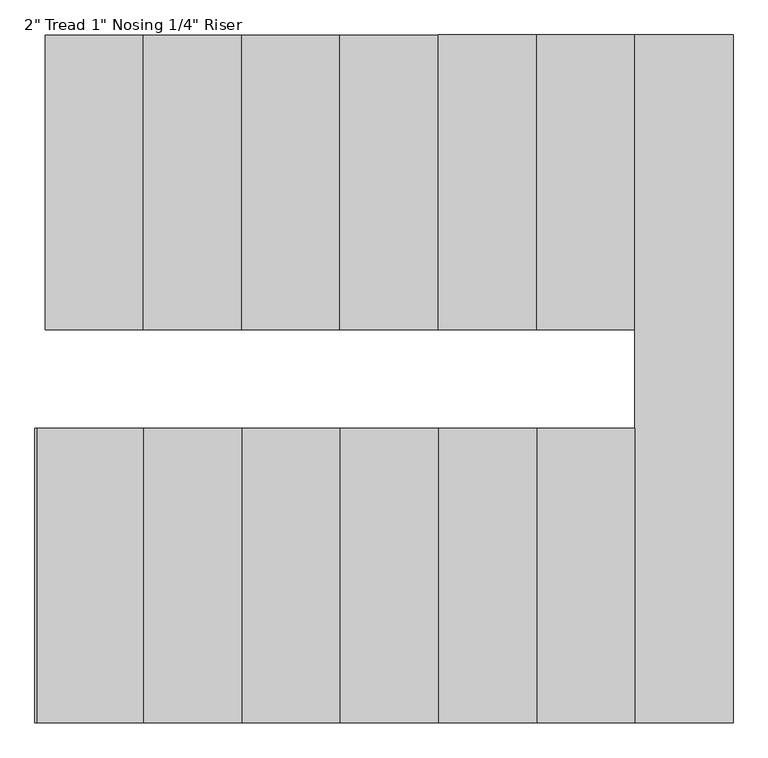
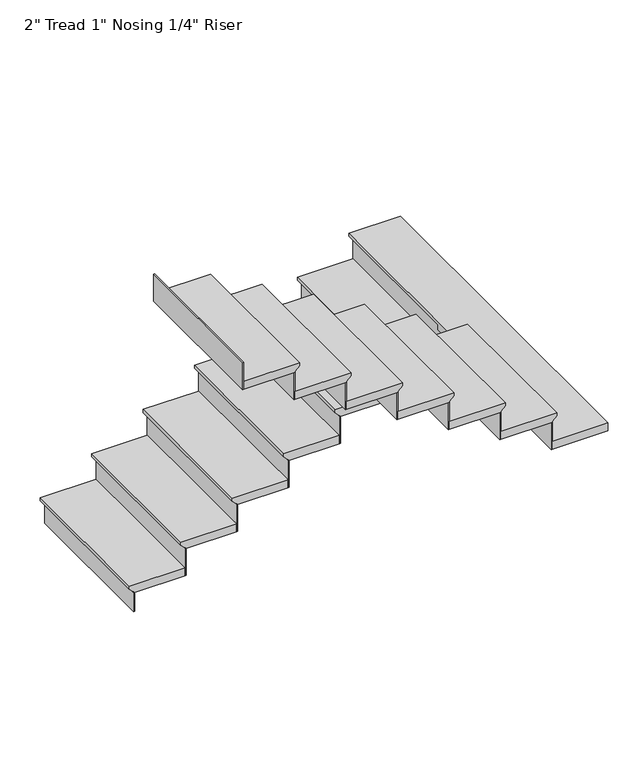
"""IFC4 building model written with IfcOpenShell, lengths in millimetres: stair flight geometry."""

from ifc_helpers import new_model, si_unit, origin, place, context, project, spatial, faceted_brep, source, transform, mapped, element, save


def stair_flight_65dd4c8f(model_context):
    return source(origin(), model_context, "Body", "Brep", [
        faceted_brep([(5003.8, 8661.4, 150.2833333), (5003.8, 8661.4, 169.3333333), (5003.8, 9575.8, 169.3333333), (5003.8, 9575.8, 150.2833333), (5029.2, 8661.4, 124.8833333), (5029.2, 9575.8, 124.8833333), (5334.0, 8661.4, 169.3333333), (5334.0, 9575.8, 169.3333333), (5029.2, 9575.8, 118.5333333), (5334.0, 9575.8, 118.5333333), (5334.0, 8661.4, 118.5333333), (5029.2, 8661.4, 118.5333333)], [[[0, 1, 2, 3]], [[4, 0, 3, 5]], [[2, 1, 6, 7]], [[8, 9, 10, 11]], [[2, 7, 9, 8, 5, 3]], [[8, 11, 4, 5]], [[6, 1, 0, 4, 11, 10]], [[7, 6, 10, 9]]]),
        faceted_brep([(5029.2, 8661.4, 118.5333333), (5029.2, 8661.4, 0.0), (5035.55, 8661.4, 0.0), (5035.55, 8661.4, 118.5333333), (5029.2, 9575.8, 118.5333333), (5035.55, 9575.8, 118.5333333), (5035.55, 9575.8, 0.0), (5029.2, 9575.8, 0.0)], [[[0, 1, 2, 3]], [[4, 5, 6, 7]], [[1, 0, 4, 7]], [[2, 1, 7, 6]], [[3, 2, 6, 5]], [[0, 3, 5, 4]]]),
        faceted_brep([(5334.0, 8661.4, 287.8666667), (5334.0, 8661.4, 118.5333333), (5340.35, 8661.4, 118.5333333), (5340.35, 8661.4, 287.8666667), (5334.0, 9575.8, 287.8666667), (5340.35, 9575.8, 287.8666667), (5340.35, 9575.8, 118.5333333), (5334.0, 9575.8, 118.5333333)], [[[0, 1, 2, 3]], [[4, 5, 6, 7]], [[1, 0, 4, 7]], [[2, 1, 7, 6]], [[3, 2, 6, 5]], [[0, 3, 5, 4]]]),
        faceted_brep([(5308.6, 9575.8, 338.6666667), (5308.6, 8661.4, 338.6666667), (5638.8, 8661.4, 338.6666667), (5638.8, 9575.8, 338.6666667), (5334.0, 9575.8, 287.8666667), (5638.8, 9575.8, 287.8666667), (5638.8, 8661.4, 287.8666667), (5334.0, 8661.4, 287.8666667), (5334.0, 9575.8, 294.2166667), (5308.6, 9575.8, 319.6166667), (5334.0, 8661.4, 294.2166667), (5308.6, 8661.4, 319.6166667)], [[[0, 1, 2, 3]], [[4, 5, 6, 7]], [[0, 3, 5, 4, 8, 9]], [[4, 7, 10, 8]], [[2, 1, 11, 10, 7, 6]], [[3, 2, 6, 5]], [[11, 1, 0, 9]], [[10, 11, 9, 8]]]),
        faceted_brep([(5638.8, 8661.4, 457.2), (5638.8, 8661.4, 287.8666667), (5645.15, 8661.4, 287.8666667), (5645.15, 8661.4, 457.2), (5638.8, 9575.8, 457.2), (5645.15, 9575.8, 457.2), (5645.15, 9575.8, 287.8666667), (5638.8, 9575.8, 287.8666667)], [[[0, 1, 2, 3]], [[4, 5, 6, 7]], [[1, 0, 4, 7]], [[2, 1, 7, 6]], [[3, 2, 6, 5]], [[0, 3, 5, 4]]]),
        faceted_brep([(5613.4, 9575.8, 508.0), (5613.4, 8661.4, 508.0), (5943.6, 8661.4, 508.0), (5943.6, 9575.8, 508.0), (5638.8, 9575.8, 457.2), (5943.6, 9575.8, 457.2), (5943.6, 8661.4, 457.2), (5638.8, 8661.4, 457.2), (5638.8, 9575.8, 463.55), (5613.4, 9575.8, 488.95), (5638.8, 8661.4, 463.55), (5613.4, 8661.4, 488.95)], [[[0, 1, 2, 3]], [[4, 5, 6, 7]], [[0, 3, 5, 4, 8, 9]], [[4, 7, 10, 8]], [[2, 1, 11, 10, 7, 6]], [[3, 2, 6, 5]], [[11, 1, 0, 9]], [[10, 11, 9, 8]]]),
        faceted_brep([(5943.6, 8661.4, 626.5333333), (5943.6, 8661.4, 457.2), (5949.95, 8661.4, 457.2), (5949.95, 8661.4, 626.5333333), (5943.6, 9575.8, 626.5333333), (5949.95, 9575.8, 626.5333333), (5949.95, 9575.8, 457.2), (5943.6, 9575.8, 457.2)], [[[0, 1, 2, 3]], [[4, 5, 6, 7]], [[1, 0, 4, 7]], [[2, 1, 7, 6]], [[3, 2, 6, 5]], [[0, 3, 5, 4]]]),
        faceted_brep([(5918.2, 9575.8, 677.3333333), (5918.2, 8661.4, 677.3333333), (6248.4, 8661.4, 677.3333333), (6248.4, 9575.8, 677.3333333), (5943.6, 9575.8, 626.5333333), (6248.4, 9575.8, 626.5333333), (6248.4, 8661.4, 626.5333333), (5943.6, 8661.4, 626.5333333), (5943.6, 9575.8, 632.8833333), (5918.2, 9575.8, 658.2833333), (5943.6, 8661.4, 632.8833333), (5918.2, 8661.4, 658.2833333)], [[[0, 1, 2, 3]], [[4, 5, 6, 7]], [[0, 3, 5, 4, 8, 9]], [[4, 7, 10, 8]], [[2, 1, 11, 10, 7, 6]], [[3, 2, 6, 5]], [[11, 1, 0, 9]], [[10, 11, 9, 8]]]),
        faceted_brep([(6248.4, 8661.4, 795.8666667), (6248.4, 8661.4, 626.5333333), (6254.75, 8661.4, 626.5333333), (6254.75, 8661.4, 795.8666667), (6248.4, 9575.8, 795.8666667), (6254.75, 9575.8, 795.8666667), (6254.75, 9575.8, 626.5333333), (6248.4, 9575.8, 626.5333333)], [[[0, 1, 2, 3]], [[4, 5, 6, 7]], [[1, 0, 4, 7]], [[2, 1, 7, 6]], [[3, 2, 6, 5]], [[0, 3, 5, 4]]]),
        faceted_brep([(6223.0, 9575.8, 846.6666667), (6223.0, 8661.4, 846.6666667), (6553.2, 8661.4, 846.6666667), (6553.2, 9575.8, 846.6666667), (6248.4, 9575.8, 795.8666667), (6553.2, 9575.8, 795.8666667), (6553.2, 8661.4, 795.8666667), (6248.4, 8661.4, 795.8666667), (6248.4, 9575.8, 802.2166667), (6223.0, 9575.8, 827.6166667), (6248.4, 8661.4, 802.2166667), (6223.0, 8661.4, 827.6166667)], [[[0, 1, 2, 3]], [[4, 5, 6, 7]], [[0, 3, 5, 4, 8, 9]], [[4, 7, 10, 8]], [[2, 1, 11, 10, 7, 6]], [[3, 2, 6, 5]], [[11, 1, 0, 9]], [[10, 11, 9, 8]]]),
        faceted_brep([(6553.2, 8661.4, 965.2), (6553.2, 8661.4, 795.8666667), (6559.55, 8661.4, 795.8666667), (6559.55, 8661.4, 965.2), (6553.2, 9575.8, 965.2), (6559.55, 9575.8, 965.2), (6559.55, 9575.8, 795.8666667), (6553.2, 9575.8, 795.8666667)], [[[0, 1, 2, 3]], [[4, 5, 6, 7]], [[1, 0, 4, 7]], [[2, 1, 7, 6]], [[3, 2, 6, 5]], [[0, 3, 5, 4]]]),
        faceted_brep([(6527.8, 9575.8, 1016.0), (6527.8, 8661.4, 1016.0), (6858.0, 8661.4, 1016.0), (6858.0, 9575.8, 1016.0), (6553.2, 9575.8, 965.2), (6858.0, 9575.8, 965.2), (6858.0, 8661.4, 965.2), (6553.2, 8661.4, 965.2), (6553.2, 9575.8, 971.55), (6527.8, 9575.8, 996.95), (6553.2, 8661.4, 971.55), (6527.8, 8661.4, 996.95)], [[[0, 1, 2, 3]], [[4, 5, 6, 7]], [[0, 3, 5, 4, 8, 9]], [[4, 7, 10, 8]], [[2, 1, 11, 10, 7, 6]], [[3, 2, 6, 5]], [[11, 1, 0, 9]], [[10, 11, 9, 8]]]),
        faceted_brep([(6858.0, 8661.4, 1134.5333333), (6858.0, 8661.4, 965.2), (6864.35, 8661.4, 965.2), (6864.35, 8661.4, 1134.5333333), (6858.0, 9575.8, 1134.5333333), (6864.35, 9575.8, 1134.5333333), (6864.35, 9575.8, 965.2), (6858.0, 9575.8, 965.2)], [[[0, 1, 2, 3]], [[4, 5, 6, 7]], [[1, 0, 4, 7]], [[2, 1, 7, 6]], [[3, 2, 6, 5]], [[0, 3, 5, 4]]]),
        faceted_brep([(6807.2, 7442.2, 1185.3333333), (7137.4, 7442.2, 1185.3333333), (7137.4, 9575.8, 1185.3333333), (6832.6, 9575.8, 1185.3333333), (6832.6, 8356.6, 1185.3333333), (6807.2, 8356.6, 1185.3333333), (7137.4, 7442.2, 1134.5333333), (6807.2, 7442.2, 1134.5333333), (6807.2, 8356.6, 1134.5333333), (6832.6, 8356.6, 1134.5333333), (6832.6, 8661.4, 1134.5333333), (6858.0, 8661.4, 1134.5333333), (6858.0, 9575.8, 1134.5333333), (7137.4, 9575.8, 1134.5333333), (6858.0, 9575.8, 1140.8833333), (6832.6, 9575.8, 1166.2833333), (6858.0, 8661.4, 1140.8833333), (6832.6, 8661.4, 1166.2833333)], [[[0, 1, 2, 3, 4, 5]], [[6, 7, 8, 9, 10, 11, 12, 13]], [[1, 0, 7, 6]], [[2, 1, 6, 13]], [[3, 2, 13, 12, 14, 15]], [[12, 11, 16, 14]], [[11, 10, 17, 16]], [[4, 3, 15, 17, 10, 9]], [[5, 4, 9, 8]], [[0, 5, 8, 7]], [[15, 14, 16, 17]]]),
        faceted_brep([(6807.2, 8356.6, 1303.8666667), (6807.2, 8356.6, 1134.5333333), (6800.85, 8356.6, 1134.5333333), (6800.85, 8356.6, 1303.8666667), (6807.2, 7442.2, 1303.8666667), (6800.85, 7442.2, 1303.8666667), (6800.85, 7442.2, 1134.5333333), (6807.2, 7442.2, 1134.5333333)], [[[0, 1, 2, 3]], [[4, 5, 6, 7]], [[1, 0, 4, 7]], [[2, 1, 7, 6]], [[3, 2, 6, 5]], [[0, 3, 5, 4]]]),
        faceted_brep([(6832.6, 7442.2, 1354.6666667), (6832.6, 8356.6, 1354.6666667), (6502.4, 8356.6, 1354.6666667), (6502.4, 7442.2, 1354.6666667), (6807.2, 7442.2, 1303.8666667), (6502.4, 7442.2, 1303.8666667), (6502.4, 8356.6, 1303.8666667), (6807.2, 8356.6, 1303.8666667), (6807.2, 7442.2, 1310.2166667), (6832.6, 7442.2, 1335.6166667), (6807.2, 8356.6, 1310.2166667), (6832.6, 8356.6, 1335.6166667)], [[[0, 1, 2, 3]], [[4, 5, 6, 7]], [[0, 3, 5, 4, 8, 9]], [[4, 7, 10, 8]], [[2, 1, 11, 10, 7, 6]], [[3, 2, 6, 5]], [[11, 1, 0, 9]], [[10, 11, 9, 8]]]),
        faceted_brep([(6502.4, 8356.6, 1473.2), (6502.4, 8356.6, 1303.8666667), (6496.05, 8356.6, 1303.8666667), (6496.05, 8356.6, 1473.2), (6502.4, 7442.2, 1473.2), (6496.05, 7442.2, 1473.2), (6496.05, 7442.2, 1303.8666667), (6502.4, 7442.2, 1303.8666667)], [[[0, 1, 2, 3]], [[4, 5, 6, 7]], [[1, 0, 4, 7]], [[2, 1, 7, 6]], [[3, 2, 6, 5]], [[0, 3, 5, 4]]]),
        faceted_brep([(6527.8, 7442.2, 1524.0), (6527.8, 8356.6, 1524.0), (6197.6, 8356.6, 1524.0), (6197.6, 7442.2, 1524.0), (6502.4, 7442.2, 1473.2), (6197.6, 7442.2, 1473.2), (6197.6, 8356.6, 1473.2), (6502.4, 8356.6, 1473.2), (6502.4, 7442.2, 1479.55), (6527.8, 7442.2, 1504.95), (6502.4, 8356.6, 1479.55), (6527.8, 8356.6, 1504.95)], [[[0, 1, 2, 3]], [[4, 5, 6, 7]], [[0, 3, 5, 4, 8, 9]], [[4, 7, 10, 8]], [[2, 1, 11, 10, 7, 6]], [[3, 2, 6, 5]], [[11, 1, 0, 9]], [[10, 11, 9, 8]]]),
        faceted_brep([(6197.6, 8356.6, 1642.5333333), (6197.6, 8356.6, 1473.2), (6191.25, 8356.6, 1473.2), (6191.25, 8356.6, 1642.5333333), (6197.6, 7442.2, 1642.5333333), (6191.25, 7442.2, 1642.5333333), (6191.25, 7442.2, 1473.2), (6197.6, 7442.2, 1473.2)], [[[0, 1, 2, 3]], [[4, 5, 6, 7]], [[1, 0, 4, 7]], [[2, 1, 7, 6]], [[3, 2, 6, 5]], [[0, 3, 5, 4]]]),
        faceted_brep([(6223.0, 7442.2, 1693.3333333), (6223.0, 8356.6, 1693.3333333), (5892.8, 8356.6, 1693.3333333), (5892.8, 7442.2, 1693.3333333), (6197.6, 7442.2, 1642.5333333), (5892.8, 7442.2, 1642.5333333), (5892.8, 8356.6, 1642.5333333), (6197.6, 8356.6, 1642.5333333), (6197.6, 7442.2, 1648.8833333), (6223.0, 7442.2, 1674.2833333), (6197.6, 8356.6, 1648.8833333), (6223.0, 8356.6, 1674.2833333)], [[[0, 1, 2, 3]], [[4, 5, 6, 7]], [[0, 3, 5, 4, 8, 9]], [[4, 7, 10, 8]], [[2, 1, 11, 10, 7, 6]], [[3, 2, 6, 5]], [[11, 1, 0, 9]], [[10, 11, 9, 8]]]),
        faceted_brep([(5892.8, 8356.6, 1811.8666667), (5892.8, 8356.6, 1642.5333333), (5886.45, 8356.6, 1642.5333333), (5886.45, 8356.6, 1811.8666667), (5892.8, 7442.2, 1811.8666667), (5886.45, 7442.2, 1811.8666667), (5886.45, 7442.2, 1642.5333333), (5892.8, 7442.2, 1642.5333333)], [[[0, 1, 2, 3]], [[4, 5, 6, 7]], [[1, 0, 4, 7]], [[2, 1, 7, 6]], [[3, 2, 6, 5]], [[0, 3, 5, 4]]]),
        faceted_brep([(5918.2, 7442.2, 1862.6666667), (5918.2, 8356.6, 1862.6666667), (5588.0, 8356.6, 1862.6666667), (5588.0, 7442.2, 1862.6666667), (5892.8, 7442.2, 1811.8666667), (5588.0, 7442.2, 1811.8666667), (5588.0, 8356.6, 1811.8666667), (5892.8, 8356.6, 1811.8666667), (5892.8, 7442.2, 1818.2166667), (5918.2, 7442.2, 1843.6166667), (5892.8, 8356.6, 1818.2166667), (5918.2, 8356.6, 1843.6166667)], [[[0, 1, 2, 3]], [[4, 5, 6, 7]], [[0, 3, 5, 4, 8, 9]], [[4, 7, 10, 8]], [[2, 1, 11, 10, 7, 6]], [[3, 2, 6, 5]], [[11, 1, 0, 9]], [[10, 11, 9, 8]]]),
        faceted_brep([(5588.0, 8356.6, 1981.2), (5588.0, 8356.6, 1811.8666667), (5581.65, 8356.6, 1811.8666667), (5581.65, 8356.6, 1981.2), (5588.0, 7442.2, 1981.2), (5581.65, 7442.2, 1981.2), (5581.65, 7442.2, 1811.8666667), (5588.0, 7442.2, 1811.8666667)], [[[0, 1, 2, 3]], [[4, 5, 6, 7]], [[1, 0, 4, 7]], [[2, 1, 7, 6]], [[3, 2, 6, 5]], [[0, 3, 5, 4]]]),
        faceted_brep([(5613.4, 7442.2, 2032.0), (5613.4, 8356.6, 2032.0), (5283.2, 8356.6, 2032.0), (5283.2, 7442.2, 2032.0), (5588.0, 7442.2, 1981.2), (5283.2, 7442.2, 1981.2), (5283.2, 8356.6, 1981.2), (5588.0, 8356.6, 1981.2), (5588.0, 7442.2, 1987.55), (5613.4, 7442.2, 2012.95), (5588.0, 8356.6, 1987.55), (5613.4, 8356.6, 2012.95)], [[[0, 1, 2, 3]], [[4, 5, 6, 7]], [[0, 3, 5, 4, 8, 9]], [[4, 7, 10, 8]], [[2, 1, 11, 10, 7, 6]], [[3, 2, 6, 5]], [[11, 1, 0, 9]], [[10, 11, 9, 8]]]),
        faceted_brep([(5283.2, 8356.6, 2150.5333333), (5283.2, 8356.6, 1981.2), (5276.85, 8356.6, 1981.2), (5276.85, 8356.6, 2150.5333333), (5283.2, 7442.2, 2150.5333333), (5276.85, 7442.2, 2150.5333333), (5276.85, 7442.2, 1981.2), (5283.2, 7442.2, 1981.2)], [[[0, 1, 2, 3]], [[4, 5, 6, 7]], [[1, 0, 4, 7]], [[2, 1, 7, 6]], [[3, 2, 6, 5]], [[0, 3, 5, 4]]]),
        faceted_brep([(4978.4, 8356.6, 2319.8666667), (4978.4, 8356.6, 2150.5333333), (4972.05, 8356.6, 2150.5333333), (4972.05, 8356.6, 2319.8666667), (4978.4, 7442.2, 2319.8666667), (4972.05, 7442.2, 2319.8666667), (4972.05, 7442.2, 2150.5333333), (4978.4, 7442.2, 2150.5333333)], [[[0, 1, 2, 3]], [[4, 5, 6, 7]], [[1, 0, 4, 7]], [[2, 1, 7, 6]], [[3, 2, 6, 5]], [[0, 3, 5, 4]]]),
        faceted_brep([(5308.6, 7442.2, 2201.3333333), (5308.6, 8356.6, 2201.3333333), (4978.4, 8356.6, 2201.3333333), (4978.4, 7442.2, 2201.3333333), (5283.2, 7442.2, 2150.5333333), (4978.4, 7442.2, 2150.5333333), (4978.4, 8356.6, 2150.5333333), (5283.2, 8356.6, 2150.5333333), (5283.2, 7442.2, 2156.8833333), (5308.6, 7442.2, 2182.2833333), (5283.2, 8356.6, 2156.8833333), (5308.6, 8356.6, 2182.2833333)], [[[0, 1, 2, 3]], [[4, 5, 6, 7]], [[0, 3, 5, 4, 8, 9]], [[4, 7, 10, 8]], [[2, 1, 11, 10, 7, 6]], [[3, 2, 6, 5]], [[11, 1, 0, 9]], [[10, 11, 9, 8]]]),
    ])


if __name__ == "__main__":
    model = new_model("IFC4")
    model_context = context("Model", 3, world=origin())
    ifc_project = project(units=[si_unit("LENGTHUNIT", "METRE", prefix="MILLI")], contexts=[model_context])
    site = spatial("IfcSite", under=ifc_project)
    building = spatial("IfcBuilding", under=site)
    placement = place(None, origin())
    stair_flight_shape = stair_flight_65dd4c8f(model_context)
    element("IfcStairFlight", 1, ObjectType="2\" Tread 1\" Nosing 1/4\" Riser", at=placement, inside=building, context=model_context, shape_type="MappedRepresentation", body=[
        mapped(stair_flight_shape, transform((0.0, 0.0, 0.0), x_axis=(1.0, 0.0, 0.0), y_axis=(0.0, 1.0, 0.0), z_axis=(0.0, 0.0, 1.0))),
    ])
    save(model, "model.ifc")
